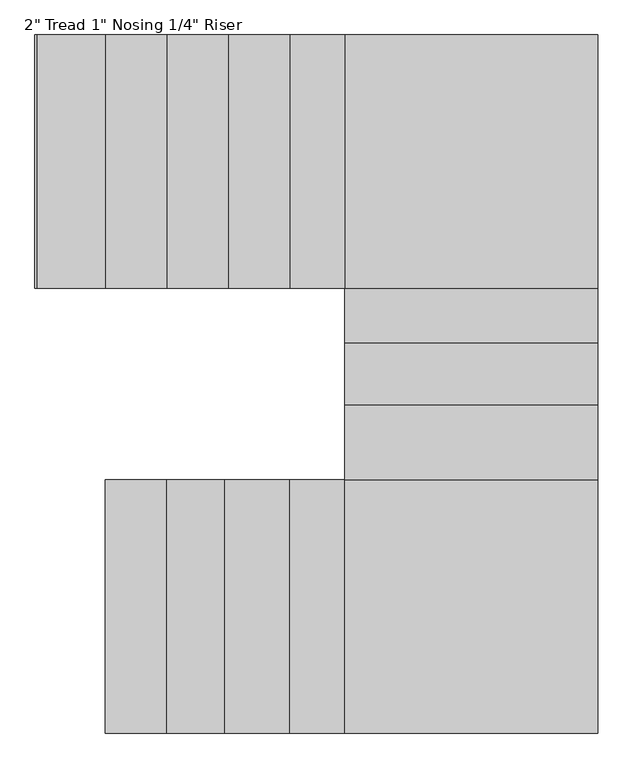
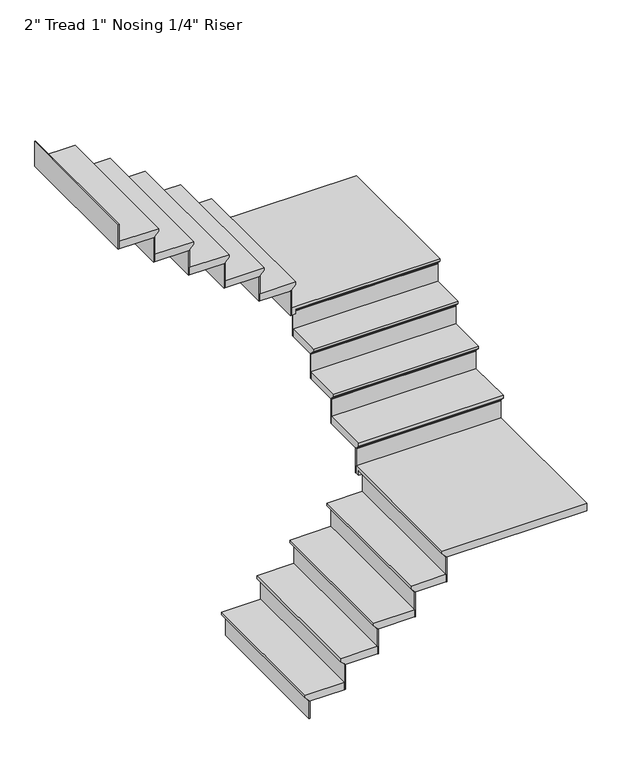
"""IFC4 building model written with IfcOpenShell, lengths in millimetres: stair flight geometry."""

from ifc_helpers import new_model, si_unit, origin, place, context, project, spatial, faceted_brep, source, transform, mapped, element, save


def stair_flight_c7955c98(model_context):
    return source(origin(), model_context, "Body", "Brep", [
        faceted_brep([(344.764115, -6141.1350571, 6551.0833333), (344.764115, -6141.1350571, 6570.1333333), (344.764115, -5201.3350571, 6570.1333333), (344.764115, -5201.3350571, 6551.0833333), (370.164115, -6141.1350571, 6525.6833333), (370.164115, -5201.3350571, 6525.6833333), (598.764115, -6141.1350571, 6570.1333333), (598.764115, -5201.3350571, 6570.1333333), (370.164115, -5201.3350571, 6519.3333333), (598.764115, -5201.3350571, 6519.3333333), (598.764115, -6141.1350571, 6519.3333333), (370.164115, -6141.1350571, 6519.3333333)], [[[0, 1, 2, 3]], [[4, 0, 3, 5]], [[2, 1, 6, 7]], [[8, 9, 10, 11]], [[2, 7, 9, 8, 5, 3]], [[8, 11, 4, 5]], [[6, 1, 0, 4, 11, 10]], [[7, 6, 10, 9]]]),
        faceted_brep([(370.164115, -6141.1350571, 6519.3333333), (370.164115, -6141.1350571, 6400.8), (376.514115, -6141.1350571, 6400.8), (376.514115, -6141.1350571, 6519.3333333), (370.164115, -5201.3350571, 6519.3333333), (376.514115, -5201.3350571, 6519.3333333), (376.514115, -5201.3350571, 6400.8), (370.164115, -5201.3350571, 6400.8)], [[[0, 1, 2, 3]], [[4, 5, 6, 7]], [[1, 0, 4, 7]], [[2, 1, 7, 6]], [[3, 2, 6, 5]], [[0, 3, 5, 4]]]),
        faceted_brep([(598.764115, -6141.1350571, 6688.6666667), (598.764115, -6141.1350571, 6519.3333333), (605.114115, -6141.1350571, 6519.3333333), (605.114115, -6141.1350571, 6688.6666667), (598.764115, -5201.3350571, 6688.6666667), (605.114115, -5201.3350571, 6688.6666667), (605.114115, -5201.3350571, 6519.3333333), (598.764115, -5201.3350571, 6519.3333333)], [[[0, 1, 2, 3]], [[4, 5, 6, 7]], [[1, 0, 4, 7]], [[2, 1, 7, 6]], [[3, 2, 6, 5]], [[0, 3, 5, 4]]]),
        faceted_brep([(573.364115, -5201.3350571, 6739.4666667), (573.364115, -6141.1350571, 6739.4666667), (814.664115, -6141.1350571, 6739.4666667), (814.664115, -5201.3350571, 6739.4666667), (598.764115, -5201.3350571, 6688.6666667), (814.664115, -5201.3350571, 6688.6666667), (814.664115, -6141.1350571, 6688.6666667), (598.764115, -6141.1350571, 6688.6666667), (598.764115, -5201.3350571, 6695.0166667), (573.364115, -5201.3350571, 6720.4166667), (598.764115, -6141.1350571, 6695.0166667), (573.364115, -6141.1350571, 6720.4166667)], [[[0, 1, 2, 3]], [[4, 5, 6, 7]], [[0, 3, 5, 4, 8, 9]], [[4, 7, 10, 8]], [[2, 1, 11, 10, 7, 6]], [[3, 2, 6, 5]], [[11, 1, 0, 9]], [[10, 11, 9, 8]]]),
        faceted_brep([(814.664115, -6141.1350571, 6858.0), (814.664115, -6141.1350571, 6688.6666667), (821.014115, -6141.1350571, 6688.6666667), (821.014115, -6141.1350571, 6858.0), (814.664115, -5201.3350571, 6858.0), (821.014115, -5201.3350571, 6858.0), (821.014115, -5201.3350571, 6688.6666667), (814.664115, -5201.3350571, 6688.6666667)], [[[0, 1, 2, 3]], [[4, 5, 6, 7]], [[1, 0, 4, 7]], [[2, 1, 7, 6]], [[3, 2, 6, 5]], [[0, 3, 5, 4]]]),
        faceted_brep([(789.264115, -5201.3350571, 6908.8), (789.264115, -6141.1350571, 6908.8), (1055.964115, -6141.1350571, 6908.8), (1055.964115, -5201.3350571, 6908.8), (814.664115, -5201.3350571, 6858.0), (1055.964115, -5201.3350571, 6858.0), (1055.964115, -6141.1350571, 6858.0), (814.664115, -6141.1350571, 6858.0), (814.664115, -5201.3350571, 6864.35), (789.264115, -5201.3350571, 6889.75), (814.664115, -6141.1350571, 6864.35), (789.264115, -6141.1350571, 6889.75)], [[[0, 1, 2, 3]], [[4, 5, 6, 7]], [[0, 3, 5, 4, 8, 9]], [[4, 7, 10, 8]], [[2, 1, 11, 10, 7, 6]], [[3, 2, 6, 5]], [[11, 1, 0, 9]], [[10, 11, 9, 8]]]),
        faceted_brep([(1055.964115, -6141.1350571, 7027.3333333), (1055.964115, -6141.1350571, 6858.0), (1062.314115, -6141.1350571, 6858.0), (1062.314115, -6141.1350571, 7027.3333333), (1055.964115, -5201.3350571, 7027.3333333), (1062.314115, -5201.3350571, 7027.3333333), (1062.314115, -5201.3350571, 6858.0), (1055.964115, -5201.3350571, 6858.0)], [[[0, 1, 2, 3]], [[4, 5, 6, 7]], [[1, 0, 4, 7]], [[2, 1, 7, 6]], [[3, 2, 6, 5]], [[0, 3, 5, 4]]]),
        faceted_brep([(1030.564115, -5201.3350571, 7078.1333333), (1030.564115, -6141.1350571, 7078.1333333), (1259.164115, -6141.1350571, 7078.1333333), (1259.164115, -5201.3350571, 7078.1333333), (1055.964115, -5201.3350571, 7027.3333333), (1259.164115, -5201.3350571, 7027.3333333), (1259.164115, -6141.1350571, 7027.3333333), (1055.964115, -6141.1350571, 7027.3333333), (1055.964115, -5201.3350571, 7033.6833333), (1030.564115, -5201.3350571, 7059.0833333), (1055.964115, -6141.1350571, 7033.6833333), (1030.564115, -6141.1350571, 7059.0833333)], [[[0, 1, 2, 3]], [[4, 5, 6, 7]], [[0, 3, 5, 4, 8, 9]], [[4, 7, 10, 8]], [[2, 1, 11, 10, 7, 6]], [[3, 2, 6, 5]], [[11, 1, 0, 9]], [[10, 11, 9, 8]]]),
        faceted_brep([(1259.164115, -6141.1350571, 7196.6666667), (1259.164115, -6141.1350571, 7027.3333333), (1265.514115, -6141.1350571, 7027.3333333), (1265.514115, -6141.1350571, 7196.6666667), (1259.164115, -5201.3350571, 7196.6666667), (1265.514115, -5201.3350571, 7196.6666667), (1265.514115, -5201.3350571, 7027.3333333), (1259.164115, -5201.3350571, 7027.3333333)], [[[0, 1, 2, 3]], [[4, 5, 6, 7]], [[1, 0, 4, 7]], [[2, 1, 7, 6]], [[3, 2, 6, 5]], [[0, 3, 5, 4]]]),
        faceted_brep([(2173.564115, -6141.1350571, 7247.4666667), (2173.564115, -5175.9350571, 7247.4666667), (1233.764115, -5175.9350571, 7247.4666667), (1233.764115, -6141.1350571, 7247.4666667), (1233.764115, -5201.3350571, 7196.6666667), (1233.764115, -5175.9350571, 7196.6666667), (2173.564115, -5175.9350571, 7196.6666667), (2173.564115, -6141.1350571, 7196.6666667), (1259.164115, -6141.1350571, 7196.6666667), (1259.164115, -5201.3350571, 7196.6666667), (1233.764115, -5201.3350571, 7228.4166667), (1233.764115, -6141.1350571, 7228.4166667), (1259.164115, -5201.3350571, 7203.0166667), (1259.164115, -6141.1350571, 7203.0166667)], [[[0, 1, 2, 3]], [[4, 5, 6, 7, 8, 9]], [[3, 2, 5, 4, 10, 11]], [[4, 9, 12, 10]], [[9, 8, 13, 12]], [[0, 3, 11, 13, 8, 7]], [[1, 0, 7, 6]], [[2, 1, 6, 5]], [[13, 11, 10, 12]]]),
        faceted_brep([(2173.564115, -5175.9350571, 7366.0), (2173.564115, -5175.9350571, 7196.6666667), (2173.564115, -5169.5850571, 7196.6666667), (2173.564115, -5169.5850571, 7366.0), (1233.764115, -5175.9350571, 7366.0), (1233.764115, -5169.5850571, 7366.0), (1233.764115, -5169.5850571, 7196.6666667), (1233.764115, -5175.9350571, 7196.6666667)], [[[0, 1, 2, 3]], [[4, 5, 6, 7]], [[1, 0, 4, 7]], [[2, 1, 7, 6]], [[3, 2, 6, 5]], [[0, 3, 5, 4]]]),
        faceted_brep([(1233.764115, -5201.3350571, 7416.8), (2173.564115, -5201.3350571, 7416.8), (2173.564115, -4896.5350571, 7416.8), (1233.764115, -4896.5350571, 7416.8), (1233.764115, -5175.9350571, 7366.0), (1233.764115, -4896.5350571, 7366.0), (2173.564115, -4896.5350571, 7366.0), (2173.564115, -5175.9350571, 7366.0), (1233.764115, -5175.9350571, 7372.35), (1233.764115, -5201.3350571, 7397.75), (2173.564115, -5175.9350571, 7372.35), (2173.564115, -5201.3350571, 7397.75)], [[[0, 1, 2, 3]], [[4, 5, 6, 7]], [[0, 3, 5, 4, 8, 9]], [[4, 7, 10, 8]], [[2, 1, 11, 10, 7, 6]], [[3, 2, 6, 5]], [[11, 1, 0, 9]], [[10, 11, 9, 8]]]),
        faceted_brep([(2173.564115, -4896.5350571, 7535.3333333), (2173.564115, -4896.5350571, 7366.0), (2173.564115, -4890.1850571, 7366.0), (2173.564115, -4890.1850571, 7535.3333333), (1233.764115, -4896.5350571, 7535.3333333), (1233.764115, -4890.1850571, 7535.3333333), (1233.764115, -4890.1850571, 7366.0), (1233.764115, -4896.5350571, 7366.0)], [[[0, 1, 2, 3]], [[4, 5, 6, 7]], [[1, 0, 4, 7]], [[2, 1, 7, 6]], [[3, 2, 6, 5]], [[0, 3, 5, 4]]]),
        faceted_brep([(1233.764115, -4921.9350571, 7586.1333333), (2173.564115, -4921.9350571, 7586.1333333), (2173.564115, -4667.9350571, 7586.1333333), (1233.764115, -4667.9350571, 7586.1333333), (1233.764115, -4896.5350571, 7535.3333333), (1233.764115, -4667.9350571, 7535.3333333), (2173.564115, -4667.9350571, 7535.3333333), (2173.564115, -4896.5350571, 7535.3333333), (1233.764115, -4896.5350571, 7541.6833333), (1233.764115, -4921.9350571, 7567.0833333), (2173.564115, -4896.5350571, 7541.6833333), (2173.564115, -4921.9350571, 7567.0833333)], [[[0, 1, 2, 3]], [[4, 5, 6, 7]], [[0, 3, 5, 4, 8, 9]], [[4, 7, 10, 8]], [[2, 1, 11, 10, 7, 6]], [[3, 2, 6, 5]], [[11, 1, 0, 9]], [[10, 11, 9, 8]]]),
        faceted_brep([(2173.564115, -4667.9350571, 7704.6666667), (2173.564115, -4667.9350571, 7535.3333333), (2173.564115, -4661.5850571, 7535.3333333), (2173.564115, -4661.5850571, 7704.6666667), (1233.764115, -4667.9350571, 7704.6666667), (1233.764115, -4661.5850571, 7704.6666667), (1233.764115, -4661.5850571, 7535.3333333), (1233.764115, -4667.9350571, 7535.3333333)], [[[0, 1, 2, 3]], [[4, 5, 6, 7]], [[1, 0, 4, 7]], [[2, 1, 7, 6]], [[3, 2, 6, 5]], [[0, 3, 5, 4]]]),
        faceted_brep([(1233.764115, -4693.3350571, 7755.4666667), (2173.564115, -4693.3350571, 7755.4666667), (2173.564115, -4464.7350571, 7755.4666667), (1233.764115, -4464.7350571, 7755.4666667), (1233.764115, -4667.9350571, 7704.6666667), (1233.764115, -4464.7350571, 7704.6666667), (2173.564115, -4464.7350571, 7704.6666667), (2173.564115, -4667.9350571, 7704.6666667), (1233.764115, -4667.9350571, 7711.0166667), (1233.764115, -4693.3350571, 7736.4166667), (2173.564115, -4667.9350571, 7711.0166667), (2173.564115, -4693.3350571, 7736.4166667)], [[[0, 1, 2, 3]], [[4, 5, 6, 7]], [[0, 3, 5, 4, 8, 9]], [[4, 7, 10, 8]], [[2, 1, 11, 10, 7, 6]], [[3, 2, 6, 5]], [[11, 1, 0, 9]], [[10, 11, 9, 8]]]),
        faceted_brep([(2173.564115, -4464.7350571, 7874.0), (2173.564115, -4464.7350571, 7704.6666667), (2173.564115, -4458.3850571, 7704.6666667), (2173.564115, -4458.3850571, 7874.0), (1233.764115, -4464.7350571, 7874.0), (1233.764115, -4458.3850571, 7874.0), (1233.764115, -4458.3850571, 7704.6666667), (1233.764115, -4464.7350571, 7704.6666667)], [[[0, 1, 2, 3]], [[4, 5, 6, 7]], [[1, 0, 4, 7]], [[2, 1, 7, 6]], [[3, 2, 6, 5]], [[0, 3, 5, 4]]]),
        faceted_brep([(2173.564115, -3550.3350571, 7924.8), (1208.364115, -3550.3350571, 7924.8), (1208.364115, -4490.1350571, 7924.8), (2173.564115, -4490.1350571, 7924.8), (1233.764115, -4490.1350571, 7874.0), (1208.364115, -4490.1350571, 7874.0), (1208.364115, -3550.3350571, 7874.0), (2173.564115, -3550.3350571, 7874.0), (2173.564115, -4464.7350571, 7874.0), (1233.764115, -4464.7350571, 7874.0), (1233.764115, -4490.1350571, 7905.75), (2173.564115, -4490.1350571, 7905.75), (1233.764115, -4464.7350571, 7880.35), (2173.564115, -4464.7350571, 7880.35)], [[[0, 1, 2, 3]], [[4, 5, 6, 7, 8, 9]], [[3, 2, 5, 4, 10, 11]], [[4, 9, 12, 10]], [[9, 8, 13, 12]], [[0, 3, 11, 13, 8, 7]], [[1, 0, 7, 6]], [[2, 1, 6, 5]], [[13, 11, 10, 12]]]),
        faceted_brep([(1208.364115, -3550.3350571, 8043.3333333), (1208.364115, -3550.3350571, 7874.0), (1202.014115, -3550.3350571, 7874.0), (1202.014115, -3550.3350571, 8043.3333333), (1208.364115, -4490.1350571, 8043.3333333), (1202.014115, -4490.1350571, 8043.3333333), (1202.014115, -4490.1350571, 7874.0), (1208.364115, -4490.1350571, 7874.0)], [[[0, 1, 2, 3]], [[4, 5, 6, 7]], [[1, 0, 4, 7]], [[2, 1, 7, 6]], [[3, 2, 6, 5]], [[0, 3, 5, 4]]]),
        faceted_brep([(1233.764115, -4490.1350571, 8094.1333333), (1233.764115, -3550.3350571, 8094.1333333), (1005.164115, -3550.3350571, 8094.1333333), (1005.164115, -4490.1350571, 8094.1333333), (1208.364115, -4490.1350571, 8043.3333333), (1005.164115, -4490.1350571, 8043.3333333), (1005.164115, -3550.3350571, 8043.3333333), (1208.364115, -3550.3350571, 8043.3333333), (1208.364115, -4490.1350571, 8049.6833333), (1233.764115, -4490.1350571, 8075.0833333), (1208.364115, -3550.3350571, 8049.6833333), (1233.764115, -3550.3350571, 8075.0833333)], [[[0, 1, 2, 3]], [[4, 5, 6, 7]], [[0, 3, 5, 4, 8, 9]], [[4, 7, 10, 8]], [[2, 1, 11, 10, 7, 6]], [[3, 2, 6, 5]], [[11, 1, 0, 9]], [[10, 11, 9, 8]]]),
        faceted_brep([(1005.164115, -3550.3350571, 8212.6666667), (1005.164115, -3550.3350571, 8043.3333333), (998.814115, -3550.3350571, 8043.3333333), (998.814115, -3550.3350571, 8212.6666667), (1005.164115, -4490.1350571, 8212.6666667), (998.814115, -4490.1350571, 8212.6666667), (998.814115, -4490.1350571, 8043.3333333), (1005.164115, -4490.1350571, 8043.3333333)], [[[0, 1, 2, 3]], [[4, 5, 6, 7]], [[1, 0, 4, 7]], [[2, 1, 7, 6]], [[3, 2, 6, 5]], [[0, 3, 5, 4]]]),
        faceted_brep([(1030.564115, -4490.1350571, 8263.4666667), (1030.564115, -3550.3350571, 8263.4666667), (776.564115, -3550.3350571, 8263.4666667), (776.564115, -4490.1350571, 8263.4666667), (1005.164115, -4490.1350571, 8212.6666667), (776.564115, -4490.1350571, 8212.6666667), (776.564115, -3550.3350571, 8212.6666667), (1005.164115, -3550.3350571, 8212.6666667), (1005.164115, -4490.1350571, 8219.0166667), (1030.564115, -4490.1350571, 8244.4166667), (1005.164115, -3550.3350571, 8219.0166667), (1030.564115, -3550.3350571, 8244.4166667)], [[[0, 1, 2, 3]], [[4, 5, 6, 7]], [[0, 3, 5, 4, 8, 9]], [[4, 7, 10, 8]], [[2, 1, 11, 10, 7, 6]], [[3, 2, 6, 5]], [[11, 1, 0, 9]], [[10, 11, 9, 8]]]),
        faceted_brep([(776.564115, -3550.3350571, 8382.0), (776.564115, -3550.3350571, 8212.6666667), (770.214115, -3550.3350571, 8212.6666667), (770.214115, -3550.3350571, 8382.0), (776.564115, -4490.1350571, 8382.0), (770.214115, -4490.1350571, 8382.0), (770.214115, -4490.1350571, 8212.6666667), (776.564115, -4490.1350571, 8212.6666667)], [[[0, 1, 2, 3]], [[4, 5, 6, 7]], [[1, 0, 4, 7]], [[2, 1, 7, 6]], [[3, 2, 6, 5]], [[0, 3, 5, 4]]]),
        faceted_brep([(801.964115, -4490.1350571, 8432.8), (801.964115, -3550.3350571, 8432.8), (547.964115, -3550.3350571, 8432.8), (547.964115, -4490.1350571, 8432.8), (776.564115, -4490.1350571, 8382.0), (547.964115, -4490.1350571, 8382.0), (547.964115, -3550.3350571, 8382.0), (776.564115, -3550.3350571, 8382.0), (776.564115, -4490.1350571, 8388.35), (801.964115, -4490.1350571, 8413.75), (776.564115, -3550.3350571, 8388.35), (801.964115, -3550.3350571, 8413.75)], [[[0, 1, 2, 3]], [[4, 5, 6, 7]], [[0, 3, 5, 4, 8, 9]], [[4, 7, 10, 8]], [[2, 1, 11, 10, 7, 6]], [[3, 2, 6, 5]], [[11, 1, 0, 9]], [[10, 11, 9, 8]]]),
        faceted_brep([(547.964115, -3550.3350571, 8551.3333333), (547.964115, -3550.3350571, 8382.0), (541.614115, -3550.3350571, 8382.0), (541.614115, -3550.3350571, 8551.3333333), (547.964115, -4490.1350571, 8551.3333333), (541.614115, -4490.1350571, 8551.3333333), (541.614115, -4490.1350571, 8382.0), (547.964115, -4490.1350571, 8382.0)], [[[0, 1, 2, 3]], [[4, 5, 6, 7]], [[1, 0, 4, 7]], [[2, 1, 7, 6]], [[3, 2, 6, 5]], [[0, 3, 5, 4]]]),
        faceted_brep([(573.364115, -4490.1350571, 8602.1333333), (573.364115, -3550.3350571, 8602.1333333), (319.364115, -3550.3350571, 8602.1333333), (319.364115, -4490.1350571, 8602.1333333), (547.964115, -4490.1350571, 8551.3333333), (319.364115, -4490.1350571, 8551.3333333), (319.364115, -3550.3350571, 8551.3333333), (547.964115, -3550.3350571, 8551.3333333), (547.964115, -4490.1350571, 8557.6833333), (573.364115, -4490.1350571, 8583.0833333), (547.964115, -3550.3350571, 8557.6833333), (573.364115, -3550.3350571, 8583.0833333)], [[[0, 1, 2, 3]], [[4, 5, 6, 7]], [[0, 3, 5, 4, 8, 9]], [[4, 7, 10, 8]], [[2, 1, 11, 10, 7, 6]], [[3, 2, 6, 5]], [[11, 1, 0, 9]], [[10, 11, 9, 8]]]),
        faceted_brep([(319.364115, -3550.3350571, 8720.6666667), (319.364115, -3550.3350571, 8551.3333333), (313.014115, -3550.3350571, 8551.3333333), (313.014115, -3550.3350571, 8720.6666667), (319.364115, -4490.1350571, 8720.6666667), (313.014115, -4490.1350571, 8720.6666667), (313.014115, -4490.1350571, 8551.3333333), (319.364115, -4490.1350571, 8551.3333333)], [[[0, 1, 2, 3]], [[4, 5, 6, 7]], [[1, 0, 4, 7]], [[2, 1, 7, 6]], [[3, 2, 6, 5]], [[0, 3, 5, 4]]]),
        faceted_brep([(90.764115, -3550.3350571, 8890.0), (90.764115, -3550.3350571, 8720.6666667), (84.414115, -3550.3350571, 8720.6666667), (84.414115, -3550.3350571, 8890.0), (90.764115, -4490.1350571, 8890.0), (84.414115, -4490.1350571, 8890.0), (84.414115, -4490.1350571, 8720.6666667), (90.764115, -4490.1350571, 8720.6666667)], [[[0, 1, 2, 3]], [[4, 5, 6, 7]], [[1, 0, 4, 7]], [[2, 1, 7, 6]], [[3, 2, 6, 5]], [[0, 3, 5, 4]]]),
        faceted_brep([(344.764115, -4490.1350571, 8771.4666667), (344.764115, -3550.3350571, 8771.4666667), (90.764115, -3550.3350571, 8771.4666667), (90.764115, -4490.1350571, 8771.4666667), (319.364115, -4490.1350571, 8720.6666667), (90.764115, -4490.1350571, 8720.6666667), (90.764115, -3550.3350571, 8720.6666667), (319.364115, -3550.3350571, 8720.6666667), (319.364115, -4490.1350571, 8727.0166667), (344.764115, -4490.1350571, 8752.4166667), (319.364115, -3550.3350571, 8727.0166667), (344.764115, -3550.3350571, 8752.4166667)], [[[0, 1, 2, 3]], [[4, 5, 6, 7]], [[0, 3, 5, 4, 8, 9]], [[4, 7, 10, 8]], [[2, 1, 11, 10, 7, 6]], [[3, 2, 6, 5]], [[11, 1, 0, 9]], [[10, 11, 9, 8]]]),
    ])


if __name__ == "__main__":
    model = new_model("IFC4")
    model_context = context("Model", 3, world=origin())
    ifc_project = project(units=[si_unit("LENGTHUNIT", "METRE", prefix="MILLI")], contexts=[model_context])
    site = spatial("IfcSite", under=ifc_project)
    building = spatial("IfcBuilding", under=site)
    placement = place(None, origin())
    stair_flight_shape = stair_flight_c7955c98(model_context)
    element("IfcStairFlight", 1, ObjectType="2\" Tread 1\" Nosing 1/4\" Riser", at=placement, inside=building, context=model_context, shape_type="MappedRepresentation", body=[
        mapped(stair_flight_shape, transform((0.0, 0.0, 0.0), x_axis=(1.0, 0.0, 0.0), y_axis=(0.0, 1.0, 0.0), z_axis=(0.0, 0.0, 1.0))),
    ])
    save(model, "model.ifc")
